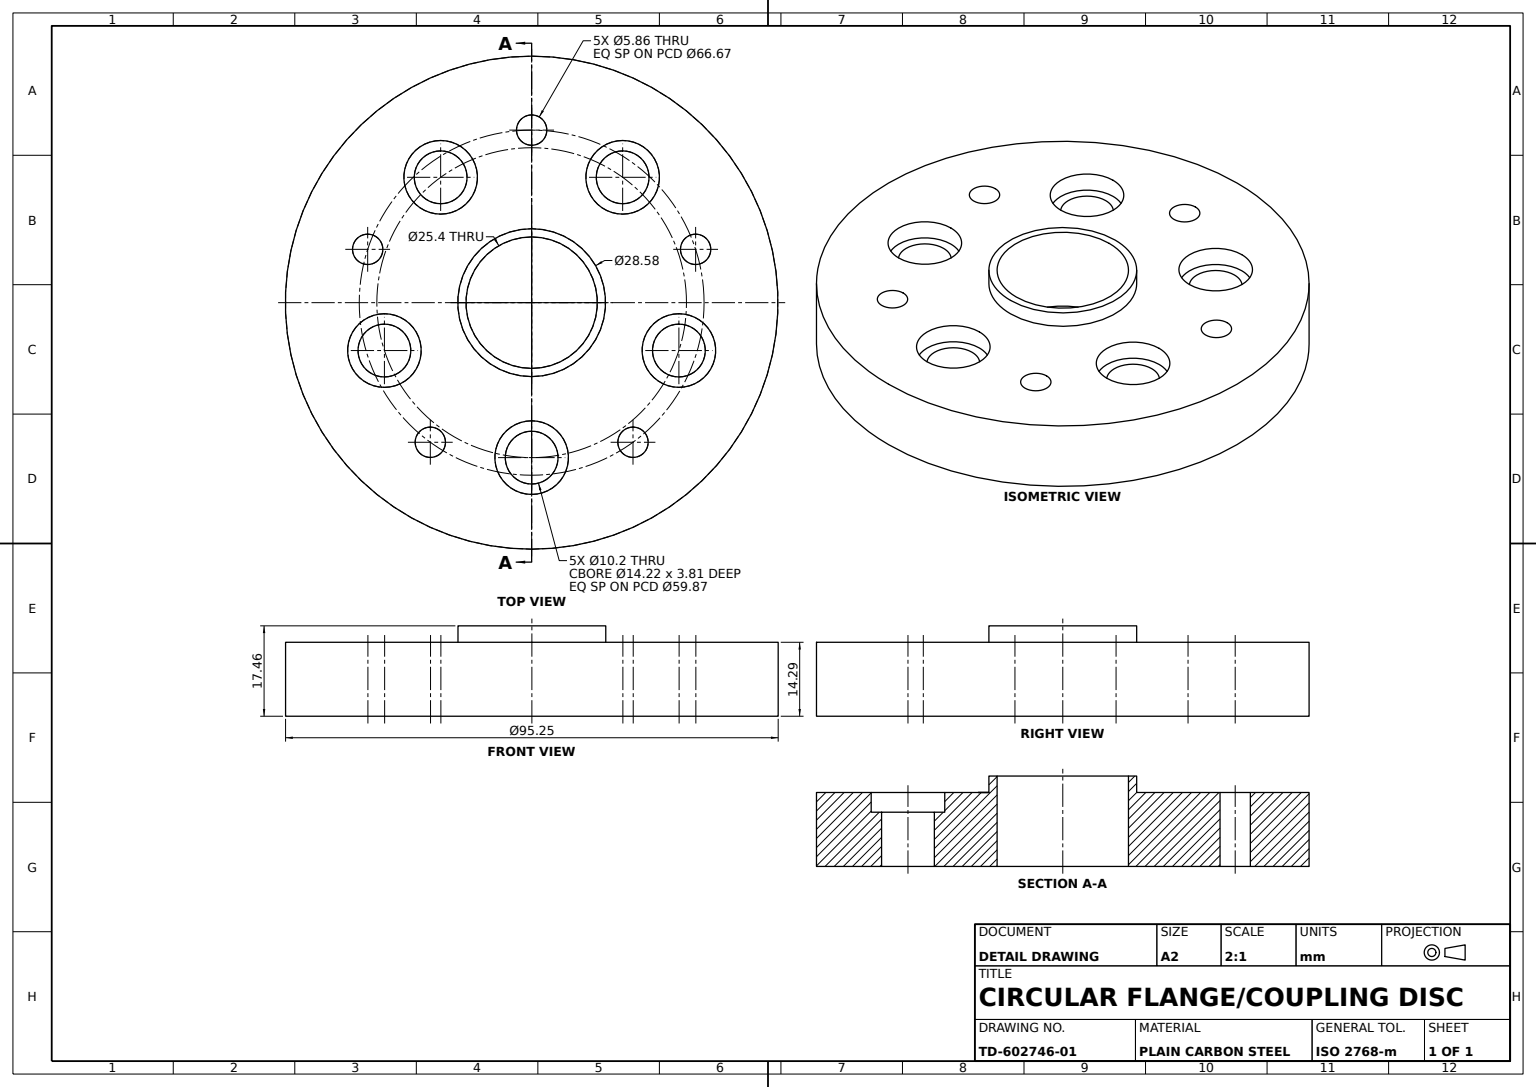
from build123d import *

# Parameters (mm, degrees)
FLANGE_DISC_SKETCH_R              = 47.625
FLANGE_DISC_3_75_DEPTH            = 14.2875
TAPPED_HOLES_SKETCH_R             = 2.930707565
TAPPED_HOLES_5X_ON_BC_2_625_DEPTH = 14.2875
HUB_BOSS_SKETCH_R                 = 14.2875
HUB_BOSS_1_125_DEPTH              = 3.175
CENTER_BORE_SKETCH_R              = 12.7
CENTER_BORE_1_0_DEPTH             = 34.925
COUNTERBORES_SKETCH_R             = 7.112
COUNTERBORES_5X_0_56_DEPTH        = 3.81
BOLT_HOLES_SKETCH_R               = 5.10197716
COUNTERBORED_BOLT_HOLES_5X_DEPTH  = 16.51


with BuildPart() as part:
    # Flange Disc Sketch → Flange Disc Ø3.75 (new body)
    with BuildSketch(Plane(origin=(0, 0, 0), x_dir=(1, 0, 0), z_dir=(0, 1, 0))):
        with Locations(Location((0, 0, 0), (0, 0, 270))):
            Circle(FLANGE_DISC_SKETCH_R)
    extrude(amount=FLANGE_DISC_3_75_DEPTH)

    # Tapped Holes Sketch → Tapped Holes 5x on BC Ø2.625 (cut)
    with BuildSketch(Plane(origin=(0, 14.2875, 0), x_dir=(1, 0, 0), z_dir=(0, 1, 0))):
        with Locations(Location((0, 33.3375, 0), (0, 0, 270))):
            Circle(TAPPED_HOLES_SKETCH_R)
        with Locations(Location((31.705846612, 10.30185405, 0), (0, 0, 270))):
            Circle(TAPPED_HOLES_SKETCH_R)
        with Locations(Location((19.595290848, -26.97060405, 0), (0, 0, 270))):
            Circle(TAPPED_HOLES_SKETCH_R)
        with Locations(Location((-19.595290848, -26.97060405, 0), (0, 0, 270))):
            Circle(TAPPED_HOLES_SKETCH_R)
        with Locations(Location((-31.705846612, 10.30185405, 0), (0, 0, 270))):
            Circle(TAPPED_HOLES_SKETCH_R)
    extrude(amount=-TAPPED_HOLES_5X_ON_BC_2_625_DEPTH, mode=Mode.SUBTRACT)

    # Hub Boss Sketch → Hub Boss Ø1.125 (add)
    with BuildSketch(Plane(origin=(0, 14.2875, 0), x_dir=(1, 0, 0), z_dir=(0, 1, 0))):
        with Locations(Location((0, 0, 0), (0, 0, 270))):
            Circle(HUB_BOSS_SKETCH_R)
    extrude(amount=HUB_BOSS_1_125_DEPTH)

    # Center Bore Sketch → Center Bore Ø1.0 (cut)
    with BuildSketch(Plane(origin=(0, 17.4625, 0), x_dir=(1, 0, 0), z_dir=(0, 1, 0))):
        with Locations(Location((0, 0, 0), (0, 0, 270))):
            Circle(CENTER_BORE_SKETCH_R)
    extrude(amount=-CENTER_BORE_1_0_DEPTH, mode=Mode.SUBTRACT)

    # Counterbores Sketch → Counterbores 5xØ0.56 (cut)
    with BuildSketch(Plane(origin=(0, 14.2875, 0), x_dir=(1, 0, 0), z_dir=(0, 1, 0))):
        with Locations(Location((0, -29.935700362, 0), (0, 0, 270))):
            Circle(COUNTERBORES_SKETCH_R)
        with Locations(Location((-28.470542899, -9.25064015, 0), (0, 0, 270))):
            Circle(COUNTERBORES_SKETCH_R)
        with Locations(Location((-17.59576319, 24.218490331, 0), (0, 0, 270))):
            Circle(COUNTERBORES_SKETCH_R)
        with Locations(Location((17.59576319, 24.218490331, 0), (0, 0, 270))):
            Circle(COUNTERBORES_SKETCH_R)
        with Locations(Location((28.470542899, -9.25064015, 0), (0, 0, 270))):
            Circle(COUNTERBORES_SKETCH_R)
    extrude(amount=-COUNTERBORES_5X_0_56_DEPTH, mode=Mode.SUBTRACT)

    # Bolt Holes Sketch → Counterbored Bolt Holes 5x (cut)
    with BuildSketch(Plane(origin=(0, 10.4775, 0), x_dir=(1, 0, 0), z_dir=(0, 1, 0))):
        with Locations(Location((0, -29.935700362, 0), (0, 0, 270))):
            Circle(BOLT_HOLES_SKETCH_R)
        with Locations(Location((-28.470542899, -9.25064015, 0), (0, 0, 270))):
            Circle(BOLT_HOLES_SKETCH_R)
        with Locations(Location((-17.59576319, 24.218490331, 0), (0, 0, 270))):
            Circle(BOLT_HOLES_SKETCH_R)
        with Locations(Location((17.59576319, 24.218490331, 0), (0, 0, 270))):
            Circle(BOLT_HOLES_SKETCH_R)
        with Locations(Location((28.470542899, -9.25064015, 0), (0, 0, 270))):
            Circle(BOLT_HOLES_SKETCH_R)
    extrude(amount=-COUNTERBORED_BOLT_HOLES_5X_DEPTH, mode=Mode.SUBTRACT)


solid = part.part
